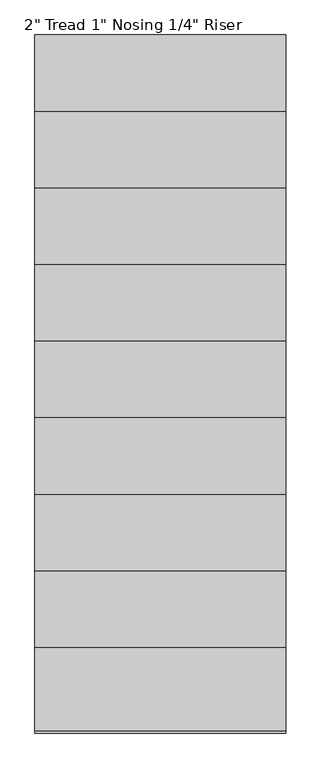
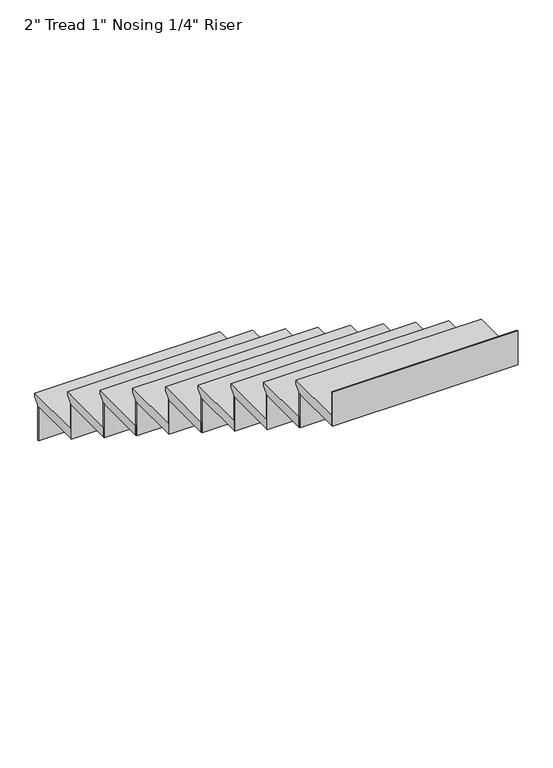
"""IFC4 building model written with IfcOpenShell, lengths in millimetres: stair flight geometry."""

from ifc_helpers import new_model, si_unit, frame, origin, place, context, project, spatial, polyline, outline, extrude, source, transform, mapped, element, save


def stair_flight_b4f684d8(model_context):
    return source(origin(), model_context, "Body", "SweptSolid", [
        extrude(outline(polyline([(1808.6257925, 5410.2), (2113.4257925, 5410.2), (2113.4257925, 5391.15), (2088.0257925, 5365.75), (2088.0257925, 5359.4), (1808.6257925, 5359.4), (1808.6257925, 5410.2)])), frame((1465.4501403, 0.0, 0.0), z_axis=(1.0, 0.0, 0.0), x_axis=(0.0, 1.0, 0.0)), (0.0, 0.0, 1.0), 914.4),
        extrude(outline(polyline([(1465.4501403, 2081.6757925), (1465.4501403, 2088.0257925), (2379.8501403, 2088.0257925), (2379.8501403, 2081.6757925), (1465.4501403, 2081.6757925)])), frame((0.0, 0.0, 5181.6), z_axis=(0.0, 0.0, 1.0), x_axis=(1.0, 0.0, 0.0)), (0.0, 0.0, 1.0), 177.8),
        extrude(outline(polyline([(1465.4501403, 1802.2757925), (1465.4501403, 1808.6257925), (2379.8501403, 1808.6257925), (2379.8501403, 1802.2757925), (1465.4501403, 1802.2757925)])), frame((0.0, 0.0, 5359.4), z_axis=(0.0, 0.0, 1.0), x_axis=(1.0, 0.0, 0.0)), (0.0, 0.0, 1.0), 177.8),
        extrude(outline(polyline([(1529.2257925, 5588.0), (1834.0257925, 5588.0), (1834.0257925, 5568.95), (1808.6257925, 5543.55), (1808.6257925, 5537.2), (1529.2257925, 5537.2), (1529.2257925, 5588.0)])), frame((1465.4501403, 0.0, 0.0), z_axis=(1.0, 0.0, 0.0), x_axis=(0.0, 1.0, 0.0)), (0.0, 0.0, 1.0), 914.4),
        extrude(outline(polyline([(1465.4501403, 1522.8757925), (1465.4501403, 1529.2257925), (2379.8501403, 1529.2257925), (2379.8501403, 1522.8757925), (1465.4501403, 1522.8757925)])), frame((0.0, 0.0, 5537.2), z_axis=(0.0, 0.0, 1.0), x_axis=(1.0, 0.0, 0.0)), (0.0, 0.0, 1.0), 177.8),
        extrude(outline(polyline([(1249.8257925, 5765.8), (1554.6257925, 5765.8), (1554.6257925, 5746.75), (1529.2257925, 5721.35), (1529.2257925, 5715.0), (1249.8257925, 5715.0), (1249.8257925, 5765.8)])), frame((1465.4501403, 0.0, 0.0), z_axis=(1.0, 0.0, 0.0), x_axis=(0.0, 1.0, 0.0)), (0.0, 0.0, 1.0), 914.4),
        extrude(outline(polyline([(1465.4501403, 1243.4757925), (1465.4501403, 1249.8257925), (2379.8501403, 1249.8257925), (2379.8501403, 1243.4757925), (1465.4501403, 1243.4757925)])), frame((0.0, 0.0, 5715.0), z_axis=(0.0, 0.0, 1.0), x_axis=(1.0, 0.0, 0.0)), (0.0, 0.0, 1.0), 177.8),
        extrude(outline(polyline([(970.4257925, 5943.6), (1275.2257925, 5943.6), (1275.2257925, 5924.55), (1249.8257925, 5899.15), (1249.8257925, 5892.8), (970.4257925, 5892.8), (970.4257925, 5943.6)])), frame((1465.4501403, 0.0, 0.0), z_axis=(1.0, 0.0, 0.0), x_axis=(0.0, 1.0, 0.0)), (0.0, 0.0, 1.0), 914.4),
        extrude(outline(polyline([(1465.4501403, 964.0757925), (1465.4501403, 970.4257925), (2379.8501403, 970.4257925), (2379.8501403, 964.0757925), (1465.4501403, 964.0757925)])), frame((0.0, 0.0, 5892.8), z_axis=(0.0, 0.0, 1.0), x_axis=(1.0, 0.0, 0.0)), (0.0, 0.0, 1.0), 177.8),
        extrude(outline(polyline([(691.0257925, 6121.4), (995.8257925, 6121.4), (995.8257925, 6102.35), (970.4257925, 6076.95), (970.4257925, 6070.6), (691.0257925, 6070.6), (691.0257925, 6121.4)])), frame((1465.4501403, 0.0, 0.0), z_axis=(1.0, 0.0, 0.0), x_axis=(0.0, 1.0, 0.0)), (0.0, 0.0, 1.0), 914.4),
        extrude(outline(polyline([(1465.4501403, 684.6757925), (1465.4501403, 691.0257925), (2379.8501403, 691.0257925), (2379.8501403, 684.6757925), (1465.4501403, 684.6757925)])), frame((0.0, 0.0, 6070.6), z_axis=(0.0, 0.0, 1.0), x_axis=(1.0, 0.0, 0.0)), (0.0, 0.0, 1.0), 177.8),
        extrude(outline(polyline([(411.6257925, 6299.2), (716.4257925, 6299.2), (716.4257925, 6280.15), (691.0257925, 6254.75), (691.0257925, 6248.4), (411.6257925, 6248.4), (411.6257925, 6299.2)])), frame((1465.4501403, 0.0, 0.0), z_axis=(1.0, 0.0, 0.0), x_axis=(0.0, 1.0, 0.0)), (0.0, 0.0, 1.0), 914.4),
        extrude(outline(polyline([(1465.4501403, 405.2757925), (1465.4501403, 411.6257925), (2379.8501403, 411.6257925), (2379.8501403, 405.2757925), (1465.4501403, 405.2757925)])), frame((0.0, 0.0, 6248.4), z_axis=(0.0, 0.0, 1.0), x_axis=(1.0, 0.0, 0.0)), (0.0, 0.0, 1.0), 177.8),
        extrude(outline(polyline([(132.2257925, 6477.0), (437.0257925, 6477.0), (437.0257925, 6457.95), (411.6257925, 6432.55), (411.6257925, 6426.2), (132.2257925, 6426.2), (132.2257925, 6477.0)])), frame((1465.4501403, 0.0, 0.0), z_axis=(1.0, 0.0, 0.0), x_axis=(0.0, 1.0, 0.0)), (0.0, 0.0, 1.0), 914.4),
        extrude(outline(polyline([(1465.4501403, 125.8757925), (1465.4501403, 132.2257925), (2379.8501403, 132.2257925), (2379.8501403, 125.8757925), (1465.4501403, 125.8757925)])), frame((0.0, 0.0, 6426.2), z_axis=(0.0, 0.0, 1.0), x_axis=(1.0, 0.0, 0.0)), (0.0, 0.0, 1.0), 177.8),
        extrude(outline(polyline([(-147.1742075, 6654.8), (157.6257925, 6654.8), (157.6257925, 6635.75), (132.2257925, 6610.35), (132.2257925, 6604.0), (-147.1742075, 6604.0), (-147.1742075, 6654.8)])), frame((1465.4501403, 0.0, 0.0), z_axis=(1.0, 0.0, 0.0), x_axis=(0.0, 1.0, 0.0)), (0.0, 0.0, 1.0), 914.4),
        extrude(outline(polyline([(1465.4501403, -153.5242075), (1465.4501403, -147.1742075), (2379.8501403, -147.1742075), (2379.8501403, -153.5242075), (1465.4501403, -153.5242075)])), frame((0.0, 0.0, 6604.0), z_axis=(0.0, 0.0, 1.0), x_axis=(1.0, 0.0, 0.0)), (0.0, 0.0, 1.0), 177.8),
        extrude(outline(polyline([(1465.4501403, -432.9242075), (1465.4501403, -426.5742075), (2379.8501403, -426.5742075), (2379.8501403, -432.9242075), (1465.4501403, -432.9242075)])), frame((0.0, 0.0, 6781.8), z_axis=(0.0, 0.0, 1.0), x_axis=(1.0, 0.0, 0.0)), (0.0, 0.0, 1.0), 177.8),
        extrude(outline(polyline([(-426.5742075, 6832.6), (-121.7742075, 6832.6), (-121.7742075, 6813.55), (-147.1742075, 6788.15), (-147.1742075, 6781.8), (-426.5742075, 6781.8), (-426.5742075, 6832.6)])), frame((1465.4501403, 0.0, 0.0), z_axis=(1.0, 0.0, 0.0), x_axis=(0.0, 1.0, 0.0)), (0.0, 0.0, 1.0), 914.4),
    ])


if __name__ == "__main__":
    model = new_model("IFC4")
    model_context = context("Model", 3, world=origin())
    ifc_project = project(units=[si_unit("LENGTHUNIT", "METRE", prefix="MILLI")], contexts=[model_context])
    site = spatial("IfcSite", under=ifc_project)
    building = spatial("IfcBuilding", under=site)
    placement = place(None, origin())
    stair_flight_shape = stair_flight_b4f684d8(model_context)
    element("IfcStairFlight", 1, ObjectType="2\" Tread 1\" Nosing 1/4\" Riser", at=placement, inside=building, context=model_context, shape_type="MappedRepresentation", body=[
        mapped(stair_flight_shape, transform((0.0, 0.0, 0.0), x_axis=(1.0, 0.0, 0.0), y_axis=(0.0, 1.0, 0.0), z_axis=(0.0, 0.0, 1.0))),
    ])
    save(model, "model.ifc")
